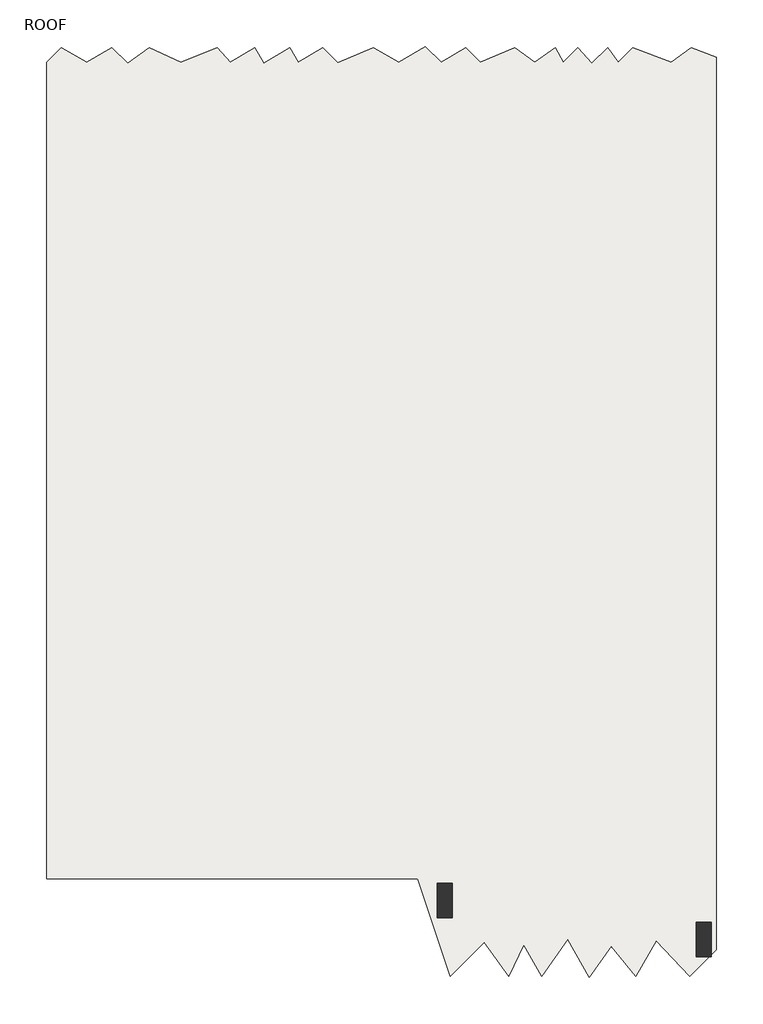
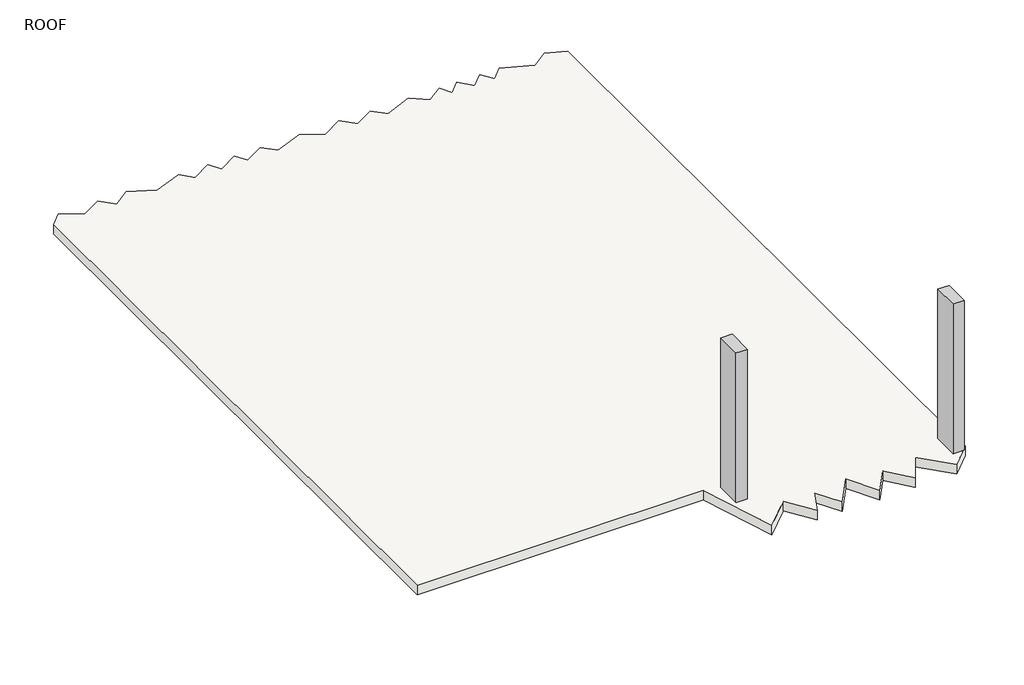
# One storey: 2 columns, 1 slab.
"""IFC4 building model written with IfcOpenShell, lengths in millimetres."""

from ifc_helpers import new_model, si_unit, frame, origin, place, context, project, spatial, polyline, outline, extrude, transform, mapped, element, save
from components import column_c97b5c1c

model = new_model("IFC4")

# Units and contexts
model_context = context("Model", 3, world=origin())
ifc_project = project(units=[si_unit("LENGTHUNIT", "METRE", prefix="MILLI")], contexts=[model_context])

# Site, building, storey
site = spatial("IfcSite", under=ifc_project)
building = spatial("IfcBuilding", under=site)
storey = spatial("IfcBuildingStorey", under=building, Name="ROOF", Elevation=9601.2)

# Columns
placement = place(None, origin())
column_shape = column_c97b5c1c(model_context)
element("IfcColumn", 1, ObjectType="Rectangular Column : x9\"", at=placement, inside=storey, context=model_context, shape_type="MappedRepresentation", body=[
    mapped(column_shape, transform((-16875.4750314, 319.9223646, 0.0), x_axis=(1.0, 0.0, 0.0), y_axis=(0.0, 1.0, 0.0), z_axis=(0.0, 0.0, 1.0))),
])
element("IfcColumn", 2, ObjectType="Rectangular Column : x9\"", at=placement, inside=storey, context=model_context, shape_type="MappedRepresentation", body=[
    mapped(column_shape, transform((-12836.8750314, -289.6776354, 0.0), x_axis=(1.0, 0.0, 0.0), y_axis=(0.0, 1.0, 0.0), z_axis=(0.0, 0.0, 1.0))),
])

# Slab
element("IfcSlab", 3, ObjectType="LW Concrete on Metal Deck", at=placement, inside=storey, context=model_context, shape_type="SweptSolid", body=[
    extrude(outline(polyline([(-23085.7750314, 13388.2223646), (-22857.1750314, 13616.8223646), (-22461.2282168, 13388.2223646), (-22065.2814022, 13616.8223646), (-21820.2943548, 13371.8353173), (-21483.0986122, 13616.8223646), (-20992.8643301, 13388.2223646), (-20427.0594754, 13616.8223646), (-20220.0943548, 13388.2223646), (-19839.6400652, 13616.8223646), (-19695.738427, 13377.3298208), (-19297.1559002, 13616.8223646), (-19159.7991627, 13388.2223646), (-18779.344873, 13616.8223646), (-18543.6943548, 13381.1718464), (-17988.5365241, 13616.8223646), (-17592.5897095, 13388.2223646), (-17180.2750314, 13635.9660173), (-16932.5313787, 13388.2223646), (-16552.077089, 13616.8223646), (-16323.477089, 13388.2223646), (-15784.9292382, 13616.8223646), (-15470.2883312, 13388.2223646), (-15155.6474241, 13616.8223646), (-15028.932375, 13388.2223646), (-14800.332375, 13616.8223646), (-14581.2943548, 13373.5559982), (-14338.0279884, 13616.8223646), (-14171.9403665, 13388.2223646), (-13943.3403665, 13616.8223646), (-13347.8170064, 13388.2223646), (-13033.1760993, 13616.8223646), (-12646.3750314, 13468.3433459), (-12646.3750314, -450.2583119), (-13057.2943548, -861.1776354), (-13577.9943548, -311.251504), (-13895.4943548, -861.1776354), (-14276.4943548, -390.1805798), (-14619.3943548, -879.8925313), (-14962.2943548, -285.9723094), (-15365.0574601, -861.1776354), (-15648.0943548, -370.9433534), (-15876.6943548, -861.1776354), (-16257.6943548, -327.7776354), (-16791.0943548, -861.1776354), (-17294.5750314, 662.8223646), (-23085.7750314, 662.8223646), (-23085.7750314, 13388.2223646)])), frame((0.0, 0.0, 9398.0), z_axis=(0.0, 0.0, 1.0), x_axis=(1.0, 0.0, 0.0)), (0.0, 0.0, 1.0), 203.2),
])

save(model, "model.ifc")

# Revit data of these elements
# Type "Rectangular Column : x9\""
#   Assembly Code = "B1010200"
#   Depth = 1' - 9"
#   Offset Base = 0' - 0"
#   Offset Top = 0' - 0"
#   Width = 0' - 9"
#   Material = none
# Type "LW Concrete on Metal Deck"
#   Assembly Code = "B1010"
#   Function = 0
#   Layers, outside or top first: 0' - 6" "Concrete, Lightweight" (function 1); 0' - 2" "Metal Deck" (function 1)
# Elements 1, 2 (IfcColumn, "Rectangular Column : x9\"")
#   Phase Created = New Construction
# Element 3 (IfcSlab, "LW Concrete on Metal Deck")
#   built-in parameter 1001955 = 0.785398 (stored number, unit not read)
#   Height Offset From Level = 0' - 0"
#   Phase Created = New Construction
#   Materials on its faces: "Metal Deck", "Concrete, Lightweight"
# Materials
#   "Concrete, Lightweight": class "Concrete", colour RGB 142 141 140, transparency 0, Description = "Lightweight concrete", Cost = 0
#   "Metal Deck": class "Metal", colour RGB 199 199 199, transparency 0, Description = "Steel, mill finish", Cost = 0
